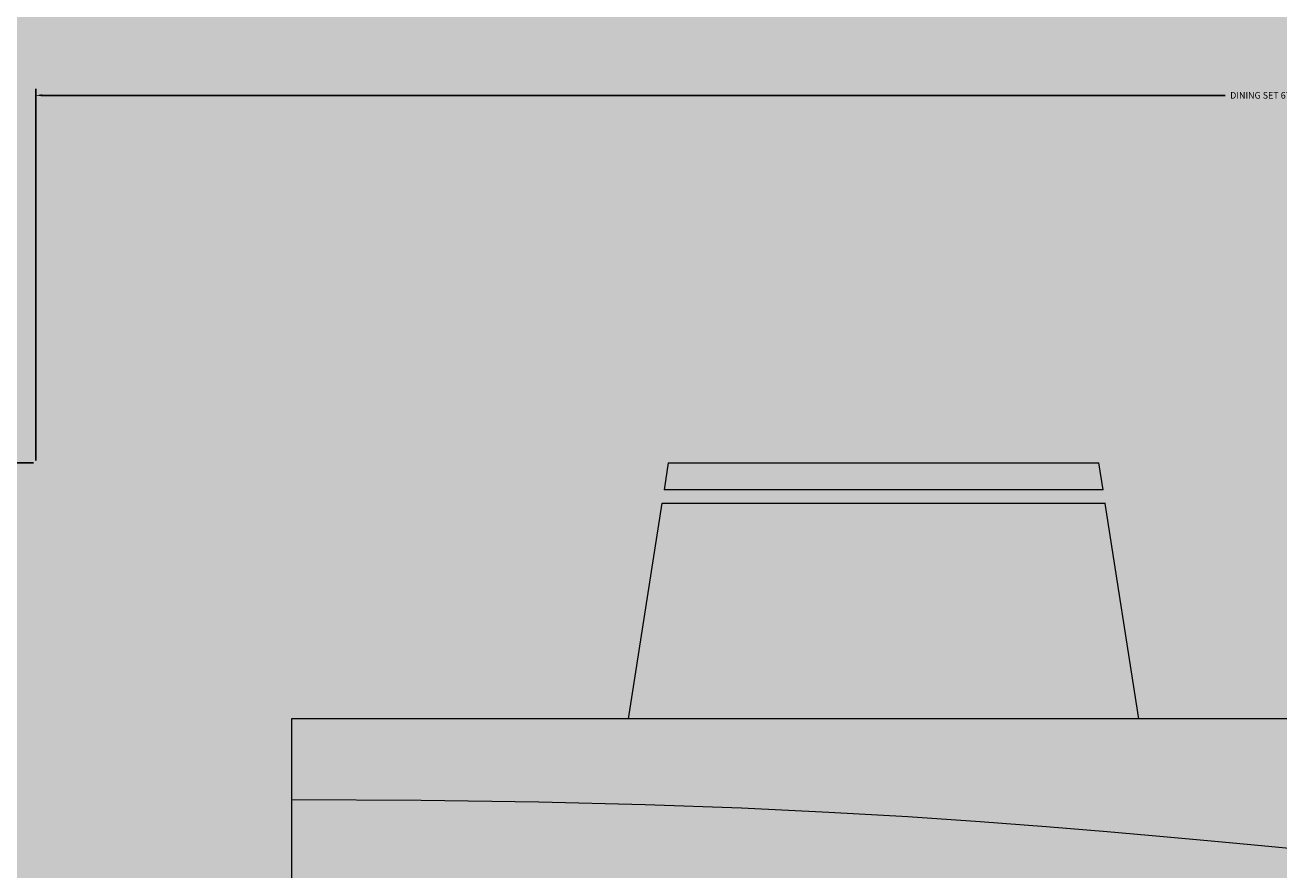
# Model space of a CAD drawing. Units: inches. Extents: x 3024 to 3952, y 1308 to 1863.
# Tile 9 of 29: x 3323 to 3357, y 1610 to 1633. Entities that reach past the tile are written whole.
import ezdxf

# ---------------------------------------------------------------- set-up
doc = ezdxf.new("R2010")
doc.units = ezdxf.units.IN
for name, color, linetype, lineweight in [('A-ANNO-DIMS', 2, 'Continuous', 18), ('A-FLOR-TILE-PATT', 7, 'Continuous', 13), ('A-FURN', 8, 'Continuous', 18), ('A-FURN-PATT', 9, 'Continuous', 13)]:
    doc.layers.add(name, color=color, linetype=linetype, lineweight=lineweight)
doc.layers.add('A-FLOR-PATT', color=254, linetype='Continuous', lineweight=13, true_color=0xfeeab9)
doc.styles.get("Standard").update_dxf_attribs({"font": 'arial.ttf'})
doc.dimstyles.get("Standard").update_dxf_attribs({"dimtxt": 0.18, "dimasz": 0.18, "dimexe": 0.18, "dimexo": 0.0625, "dimgap": 0.09, "dimtad": 0, "dimtih": 1, "dimtoh": 1, "dimdec": 4, "dimzin": 0, "dimdsep": 46, "dimtxsty": 'Standard', "dimcen": 0.09, "dimadec": 0, "dimazin": 0, "dimtfac": 1, "dimtdec": 4, "dimtofl": 0, "dimtmove": 0, "dimatfit": 3, "dimfxl": 1, "dimtolj": 1, "dimtzin": 0, "dimarcsym": 0})

# ---------------------------------------------------------------- blocks, each defined once
blk = doc.blocks.new('Dining Set - 36 x 72 in.')
for p, q in [((-22, 27.5), (-22.1562, 26.50042)), ((-22, 27.5), (-6, 27.5)), ((-5.8437, 26.49966), (-6, 27.5)), ((-5.8416, 26.5), (-22.1534, 26.5)), ((-22.2343, 26.00059), (-23.4847, 17.99762)), ((-22.2304, 26), (-5.7608, 26)), ((-4.5152, 17.99762), (-5.7655, 25.99926)), ((36, 18), (-36, 18)), ((-36, 18), (-36, -18))]:
    blk.add_line(p, q)
blk.add_lwpolyline([(-36, 15), (-31.1772, 14.97754), (-26.8079, 14.91406), (-22.8538, 14.81543), (-19.276, 14.6875), (-16.0362, 14.53613), (-13.0957, 14.36718), (-10.4159, 14.18652), (-7.9583, 14), (-5.6904, 13.81315), (-3.6035, 13.63021), (-1.6954, 13.45508), (0.0365, 13.29166), (1.5945, 13.14388)])
blk = doc.blocks.new('*D20')
at = {"layer": 'A-ANNO-DIMS', "color": 0, "lineweight": -2, "transparency": 16777216}
for p, q in [((3323.117, 1621.176), (3323.117, 1631.358)), ((3323.297, 1631.178), (3355.696, 1631.178)), ((3390.032, 1631.178), (3357.634, 1631.178)), ((3390.212, 1621.176), (3390.212, 1631.358))]:
    blk.add_line(p, q, dxfattribs=at)
at = {"layer": 'A-ANNO-DIMS', "color": 0, "transparency": 16777216}
for points in [[(3323.297, 1631.208), (3323.297, 1631.148), (3323.117, 1631.178)], [(3390.032, 1631.208), (3390.032, 1631.148), (3390.212, 1631.178)]]:
    blk.add_solid(points, dxfattribs=at)
at = {"layer": 'Defpoints', "color": 0, "transparency": 16777216}
for p in [(3390.212, 1631.178), (3323.117, 1621.114), (3390.212, 1621.114)]:
    blk.add_point(p, dxfattribs=at)
at = {"layer": 'A-ANNO-DIMS', "color": 0, "transparency": 16777216, "insert": (3356.665, 1631.178), "char_height": 0.18, "attachment_point": 5}
blk.add_mtext('\\A1;DINING SET 67', dxfattribs=at)
blk = doc.blocks.new('*D21')
at = {"layer": 'A-ANNO-DIMS', "color": 0, "lineweight": -2, "transparency": 16777216}
for p, q in [((3323.055, 1621.114), (3312.873, 1621.114)), ((3313.053, 1620.934), (3313.053, 1601.018)), ((3313.053, 1580.742), (3313.053, 1600.657)), ((3323.055, 1580.562), (3312.873, 1580.562))]:
    blk.add_line(p, q, dxfattribs=at)
at = {"layer": 'A-ANNO-DIMS', "color": 0, "transparency": 16777216}
for points in [[(3313.023, 1620.934), (3313.083, 1620.934), (3313.053, 1621.114)], [(3313.023, 1580.742), (3313.083, 1580.742), (3313.053, 1580.562)]]:
    blk.add_solid(points, dxfattribs=at)
at = {"layer": 'Defpoints', "color": 0, "transparency": 16777216}
for p in [(3313.053, 1621.114), (3323.117, 1621.114), (3323.117, 1580.562)]:
    blk.add_point(p, dxfattribs=at)
at = {"layer": 'A-ANNO-DIMS', "color": 0, "transparency": 16777216, "insert": (3313.053, 1600.838), "char_height": 0.18, "attachment_point": 5}
blk.add_mtext('\\A1;41', dxfattribs=at)

msp = doc.modelspace()

# ---------------------------------------------------------------- hatches: boundary and pattern name
at = {"layer": 'A-FLOR-PATT', "transparency": 33554528}
h = msp.add_hatch(color=256, dxfattribs=at)
h.dxf.hatch_style = 1
h.paths.add_polyline_path([(3460.764, 1688.6064), (3412.764, 1688.6064), (3412.764, 1694.6064), (3460.764, 1694.6064), (3460.764, 1778.6064), (3406.764, 1778.6064), (3406.764, 1759.9514), (3318.2981, 1759.9514), (3318.2981, 1658.6064), (3322.5356, 1658.6064), (3322.5356, 1652.6064), (3292.764, 1652.6064), (3292.764, 1778.6064), (3106.764, 1778.6064), (3106.764, 1628.6064), (3172.764, 1628.6064), (3172.764, 1532.6064), (3166.764, 1532.6064), (3166.764, 1628.6064), (3106.764, 1628.6064), (3106.764, 1356.8452), (3202.812, 1356.8452), (3202.812, 1354.2534), (3202.812, 1353.8388), (3202.812, 1351.1212), (3202.812, 1347.8452), (3277.764, 1347.8452), (3277.764, 1353.8452), (3277.764, 1356.8452), (3277.764, 1442.6064), (3460.764, 1442.6064)])
h.paths.add_polyline_path([(3216.238, 1527.2064), (3216.238, 1491.2064), (3214.663, 1491.2064), (3214.663, 1491.2409, -0.3966224), (3180.243, 1526.6064), (3163.0285, 1526.6064), (3163.0285, 1531.1064), (3161.716, 1531.1064), (3161.716, 1561.1064), (3163.0285, 1561.1064), (3163.0285, 1531.1064), (3163.0285, 1526.6064), (3180.243, 1526.6064, 0.3966224), (3214.663, 1491.2409), (3214.663, 1527.2064)], flags=16)
h.paths.add_polyline_path([(3227.364, 1649.8972), (3191.364, 1649.8972), (3191.364, 1651.4722), (3227.364, 1651.4722)], flags=16)
h.paths.add_polyline_path([(3323.1172, 1606.7362), (3323.8545, 1606.8514), (3323.8545, 1594.8241), (3323.1172, 1594.9393)], flags=16)
h.paths.add_polyline_path([(3324.2232, 1606.909), (3330.1216, 1607.8307), (3330.1216, 1614.1093), (3339.3495, 1614.1093), (3340.2711, 1620.0078), (3352.4136, 1620.0078), (3353.3353, 1614.1093), (3359.9941, 1614.1093), (3360.9157, 1620.0078), (3373.0582, 1620.0078), (3373.9799, 1614.1093), (3383.2077, 1614.1093), (3383.2077, 1607.8307), (3389.1062, 1606.909), (3389.1062, 1594.7665), (3383.2077, 1593.8449), (3383.2077, 1587.5663), (3373.9799, 1587.5663), (3373.0583, 1581.6678), (3360.9157, 1581.6678), (3359.9941, 1587.5663), (3353.3353, 1587.5663), (3352.4136, 1581.6678), (3340.2711, 1581.6678), (3339.3495, 1587.5663), (3330.1216, 1587.5663), (3330.1216, 1593.8449), (3324.2232, 1594.7665)], flags=16)
h.paths.add_polyline_path([(3236.1584, 1693.1064), (3236.1584, 1723.1064), (3237.4709, 1723.1064), (3237.4709, 1693.1064)], flags=16)
h.paths.add_polyline_path([(3373.2158, 1600.6847), (3373.7965, 1600.7303), (3374.3268, 1600.7874), (3374.8132, 1600.8531), (3375.2621, 1600.9247), (3375.6801, 1600.9991), (3376.0736, 1601.0735), (3376.6855, 1601.19), (3377.366, 1601.3023), (3378.0667, 1601.3814), (3378.8026, 1601.4123), (3379.5865, 1601.3839), (3380.4537, 1601.2948), (3381.301, 1601.1717), (3382.0317, 1601.0433), (3382.4398, 1600.9607), (3382.6252, 1600.9201), (3382.919, 1600.8507), (3382.9044, 1600.8531), (3382.842, 1600.8678), (3382.7541, 1600.8896), (3382.6252, 1600.9201), (3382.4398, 1600.9607), (3382.1868, 1601.0119), (3381.8738, 1601.0711), (3381.5125, 1601.1346), (3381.1149, 1601.1988), (3380.6928, 1601.2601), (3380.2581, 1601.3149), (3379.8226, 1601.3597), (3379.3984, 1601.3908), (3378.9944, 1601.4054), (3378.6092, 1601.4042), (3378.2384, 1601.3886), (3377.8777, 1601.36), (3377.5227, 1601.32), (3377.1691, 1601.2698), (3376.8127, 1601.211), (3376.4491, 1601.145), (3376.0736, 1601.0735), (3375.4177, 1600.9494), (3374.5542, 1600.8119), (3373.5044, 1600.6988)], flags=0)
h.paths.add_polyline_path([(3380.0253, 1596.7351), (3380.499, 1596.6659), (3380.9706, 1596.6119), (3381.4375, 1596.5791), (3381.8971, 1596.5736), (3382.5886, 1596.6167), (3382.7848, 1596.6692), (3382.1465, 1596.5706), (3381.236, 1596.5815), (3380.3199, 1596.6865)], flags=0)
h.paths.add_polyline_path([(3369.6414, 1603.9617), (3370.1589, 1604.0021), (3370.6218, 1604.0539), (3371.0335, 1604.1173), (3371.3978, 1604.1921), (3371.7181, 1604.2785), (3371.9984, 1604.3761), (3372.2441, 1604.483), (3372.4611, 1604.5972), (3372.655, 1604.7163), (3372.8317, 1604.8384), (3372.9968, 1604.9611), (3373.3703, 1605.2455), (3373.8426, 1605.5328), (3374.4624, 1605.7539), (3375.1058, 1605.8302), (3375.7221, 1605.8261), (3376.4109, 1605.76), (3377.1534, 1605.6376), (3377.8945, 1605.473), (3378.1382, 1605.409), (3377.7394, 1605.5074), (3377.3509, 1605.5937), (3376.9704, 1605.6677), (3376.5999, 1605.7288), (3376.2417, 1605.7762), (3375.8979, 1605.8092), (3375.5707, 1605.8271), (3375.2621, 1605.8291), (3374.9745, 1605.8146), (3374.7092, 1605.7832), (3374.4647, 1605.7359), (3374.239, 1605.6742), (3374.0298, 1605.5996), (3373.835, 1605.5134), (3373.6525, 1605.4171), (3373.4801, 1605.3123), (3373.3156, 1605.2002), (3373.1562, 1605.0825), (3372.7603, 1604.781), (3372.236, 1604.4588), (3371.5738, 1604.2283), (3370.8493, 1604.0794), (3369.9262, 1603.976)], flags=0)
h.paths.add_polyline_path([(3366.7533, 1606.5832), (3367.1713, 1606.5519), (3367.5378, 1606.5374), (3367.8568, 1606.5394), (3368.1325, 1606.5573), (3368.3694, 1606.5903), (3368.5717, 1606.6377), (3368.7438, 1606.6988), (3368.89, 1606.7728), (3369.0146, 1606.8591), (3369.121, 1606.9568), (3369.2094, 1607.0646), (3369.2792, 1607.181), (3369.3295, 1607.3046), (3369.3596, 1607.4339), (3369.3688, 1607.5676), (3369.3565, 1607.7042), (3369.3218, 1607.8422), (3369.2649, 1607.9804), (3369.1893, 1608.1187), (3369.0993, 1608.2569), (3368.9992, 1608.3952), (3368.8934, 1608.5334), (3368.7861, 1608.6717), (3368.6817, 1608.8099), (3368.4212, 1609.1804), (3368.2685, 1609.7106), (3368.4883, 1610.1814), (3369.0537, 1610.4604), (3369.6717, 1610.5097), (3370.2812, 1610.3612), (3370.4805, 1610.2968), (3370.1882, 1610.3839), (3369.9284, 1610.4472), (3369.6905, 1610.4842), (3369.4662, 1610.4933), (3369.2555, 1610.4765), (3369.0608, 1610.4367), (3368.884, 1610.3767), (3368.7274, 1610.2994), (3368.5931, 1610.2077), (3368.4833, 1610.1045), (3368.4002, 1609.9927), (3368.3451, 1609.8747), (3368.3166, 1609.7517), (3368.3127, 1609.6244), (3368.331, 1609.4935), (3368.3696, 1609.3597), (3368.4261, 1609.2237), (3368.4985, 1609.0863), (3368.5845, 1608.9482), (3368.6817, 1608.8099), (3368.7861, 1608.6717), (3368.8934, 1608.5334), (3368.9992, 1608.3952), (3369.0993, 1608.2569), (3369.3398, 1607.8876), (3369.3941, 1607.2896), (3368.9774, 1606.7817), (3368.3928, 1606.5742), (3367.7162, 1606.5303), (3367.0044, 1606.5585)], flags=0)
h.paths.add_polyline_path([(3362.1859, 1610.2589), (3362.5478, 1610.2845), (3362.8348, 1610.3275), (3363.0585, 1610.3863), (3363.2303, 1610.4595), (3363.3619, 1610.5457), (3363.463, 1610.6432), (3363.5376, 1610.7502), (3363.5876, 1610.8643), (3363.6153, 1610.9834), (3363.6229, 1611.1055), (3363.6125, 1611.2283), (3363.5861, 1611.3496), (3363.5462, 1611.4673), (3363.4949, 1611.5797), (3363.4358, 1611.6871), (3363.3723, 1611.7902), (3363.3081, 1611.8897), (3363.2468, 1611.9863), (3363.192, 1612.0808), (3363.0258, 1612.4261), (3363.3371, 1612.8672), (3363.9008, 1612.9782), (3364.4822, 1612.9641), (3365.1098, 1612.9074), (3365.328, 1612.8805), (3364.9615, 1612.9208), (3364.6426, 1612.9496), (3364.3668, 1612.9669), (3364.1299, 1612.9726), (3363.9276, 1612.9669), (3363.7555, 1612.9496), (3363.6093, 1612.9208), (3363.4848, 1612.8805), (3363.3782, 1612.8289), (3363.2889, 1612.7672), (3363.2169, 1612.6969), (3363.1622, 1612.6193), (3363.1247, 1612.5361), (3363.1046, 1612.4484), (3363.1017, 1612.358), (3363.1161, 1612.266), (3363.1472, 1612.1738), (3363.192, 1612.0808), (3363.2468, 1611.9863), (3363.3081, 1611.8897), (3363.3723, 1611.7902), (3363.4358, 1611.6871), (3363.6363, 1611.323), (3363.5979, 1610.7003), (3363.0863, 1610.3651), (3362.3983, 1610.2622)], flags=0)
h.paths.add_polyline_path([(3352.356, 1581.2991), (3352.2408, 1580.5618), (3340.4439, 1580.5618), (3340.3287, 1581.2991)], flags=16)
h.paths.add_polyline_path([(3340.4439, 1621.1137), (3352.2408, 1621.1137), (3352.356, 1620.3764), (3340.3287, 1620.3764)], flags=16)
h.paths.add_polyline_path([(3278.4282, 1504.7424), (3290.3831, 1504.7424), (3290.3831, 1502.7499), (3291.0473, 1502.7499), (3291.0473, 1494.7799), (3290.3831, 1494.7799), (3290.3831, 1494.1158), (3291.0473, 1494.1158), (3291.0473, 1486.1458), (3290.3831, 1486.1458), (3290.3831, 1484.1533), (3291.0473, 1484.1533), (3291.0473, 1483.4892, -0.0909091), (3291.0473, 1468.8776), (3291.0473, 1468.2135), (3290.3831, 1468.2135), (3290.3831, 1464.8926), (3278.4282, 1464.8926), (3278.4282, 1472.8626), (3277.764, 1473.5268), (3277.764, 1478.84), (3278.4282, 1479.5042)], flags=16)
h.paths.add_polyline_path([(3278.7603, 1504.4103), (3290.051, 1504.4103), (3290.051, 1465.2247), (3278.7603, 1465.2247)], flags=0)
h.paths.add_polyline_path([(3123.904, 1600.7821), (3117.9039, 1602.7821), (3117.9039, 1599.7821), (3119.4039, 1599.7821), (3119.4039, 1596.7821), (3118.4039, 1596.7821), (3118.4039, 1598.7821), (3117.9039, 1598.7821), (3117.9039, 1596.2821), (3109.9039, 1596.2821), (3109.9039, 1617.2821), (3117.9039, 1617.2821), (3117.9039, 1610.7821), (3123.9038, 1612.7821, -0.7025712), (3137.9039, 1606.7822, -0.7025621)], flags=16)
h.paths.add_polyline_path([(3123.9039, 1602.7822), (3123.9039, 1610.7822, -0.7345333), (3136.9039, 1606.7822, -0.7345297)], flags=0)
h.paths.add_polyline_path([(3177.972, 1689.6473), (3109.2405, 1689.6473), (3109.2405, 1741.1959), (3177.972, 1741.1959)], flags=16)
h.paths.add_polyline_path([(3373.0006, 1581.2991), (3372.8854, 1580.5618), (3361.0885, 1580.5618), (3360.9733, 1581.2991)], flags=16)
h.paths.add_polyline_path([(3361.0885, 1621.1137), (3372.8854, 1621.1137), (3373.0006, 1620.3764), (3360.9733, 1620.3764)], flags=16)
h.paths.add_polyline_path([(3116.9039, 1598.2821, -0.4142136), (3116.1539, 1597.2821), (3111.9039, 1597.2821, -0.4142136), (3110.9039, 1598.0321), (3110.9039, 1615.2821, -0.4142136), (3111.6539, 1616.2821), (3115.9039, 1616.2821, -0.4142136), (3116.9039, 1615.5321)], flags=0)
h.paths.add_polyline_path([(3121.6122, 1728.1369), (3121.6122, 1696.5205), (3110.2715, 1696.5205), (3110.2715, 1714.3906), (3121.6122, 1714.3906), (3121.6122, 1716.4526), (3110.2715, 1716.4526), (3110.2715, 1734.3228), (3123.3304, 1734.3228), (3123.3304, 1729.8552), (3134.6711, 1741.1959), (3134.6711, 1728.1369)], flags=0)
h.paths.add_polyline_path([(3389.4748, 1606.8514), (3390.2122, 1606.7362), (3390.2122, 1594.9393), (3389.4748, 1594.8241)], flags=16)
h.paths.add_polyline_path([(3257.6842, 1762.8281), (3259.6842, 1768.8281), (3256.6842, 1768.8281), (3256.6842, 1767.3281), (3253.6842, 1767.3281), (3253.6842, 1768.3281), (3255.6842, 1768.3281), (3255.6842, 1768.8281), (3253.1842, 1768.8281), (3253.1842, 1776.8281), (3274.1842, 1776.8281), (3274.1842, 1768.8281), (3267.6842, 1768.8281), (3269.6842, 1762.8282, -0.7025712), (3263.6843, 1748.8282, -0.7025621)], flags=16)
h.paths.add_polyline_path([(3259.6842, 1762.8281), (3267.6843, 1762.8281, -0.7345333), (3263.6842, 1749.8282, -0.7345297)], flags=0)
h.paths.add_polyline_path([(3411.264, 1715.6064), (3411.264, 1716.9189), (3441.264, 1716.9189), (3441.264, 1715.6064)], flags=16)
h.paths.add_polyline_path([(3178.3806, 1449.1876), (3178.3806, 1397.639), (3109.6491, 1397.639), (3109.6491, 1449.1876)], flags=16)
h.paths.add_polyline_path([(3397.1501, 1541.7146), (3419.6183, 1541.7146), (3419.6183, 1496.7783), (3397.1501, 1496.7783)], flags=16)
h.paths.add_polyline_path([(3254.1842, 1770.5781), (3254.1842, 1774.8281, -0.4142136), (3254.9342, 1775.8281), (3272.1842, 1775.8281, -0.4142136), (3273.1842, 1775.0781), (3273.1842, 1770.8281, -0.4142136), (3272.4342, 1769.8281), (3255.1842, 1769.8281, -0.4142136)], flags=0)
h.paths.add_polyline_path([(3403.672, 1500.7601), (3403.6016, 1500.3997), (3403.5328, 1500.0441), (3403.4662, 1499.6867), (3403.4027, 1499.3226), (3403.3464, 1498.9532), (3403.3025, 1498.5811), (3403.2759, 1498.2091), (3403.2714, 1497.8401), (3403.3064, 1497.2813), (3403.3491, 1497.1219), (3403.2689, 1497.6395), (3403.2778, 1498.3719), (3403.3635, 1499.0984), (3403.4889, 1499.8168), (3403.6016, 1500.3997), (3403.672, 1500.7601), (3403.744, 1501.1315), (3403.817, 1501.5205), (3403.891, 1501.9336), (3403.9656, 1502.3769), (3404.0404, 1502.8572), (3404.115, 1503.3786), (3404.2264, 1504.2311), (3404.2571, 1504.5223), (3404.1552, 1503.6598), (3404.0063, 1502.6193), (3403.8604, 1501.7518), (3403.744, 1501.1315)], flags=0)
h.paths.add_polyline_path([(3406.5868, 1505.0416), (3406.6121, 1504.5236), (3406.6492, 1504.0526), (3406.6956, 1503.624), (3406.7491, 1503.2333), (3406.8072, 1502.8759), (3406.8676, 1502.5473), (3406.9281, 1502.243), (3407.0268, 1501.7597), (3407.1416, 1501.1368), (3407.2087, 1500.3904), (3407.1804, 1499.6703), (3407.1078, 1498.9956), (3407.0074, 1498.3199), (3406.8809, 1497.6059), (3406.7403, 1496.9627), (3406.7418, 1496.9824), (3406.7491, 1497.0249), (3406.8229, 1497.3409), (3406.8364, 1497.4025), (3406.878, 1497.6078), (3406.9261, 1497.8614), (3406.9777, 1498.1526), (3407.0298, 1498.4712), (3407.0797, 1498.8068), (3407.1243, 1499.149), (3407.1607, 1499.4874), (3407.1859, 1499.8115), (3407.1978, 1500.1137), (3407.1969, 1500.3962), (3407.1841, 1500.6642), (3407.1609, 1500.9225), (3407.1284, 1501.1761), (3407.0876, 1501.43), (3407.0398, 1501.6891), (3406.9862, 1501.9585), (3406.8832, 1502.4628), (3406.7712, 1503.0713), (3406.6657, 1503.8424), (3406.5924, 1504.7735)], flags=0)
h.paths.add_polyline_path([(3409.2517, 1507.8962), (3409.2752, 1507.4282), (3409.3079, 1507.0076), (3409.3501, 1506.6314), (3409.4015, 1506.2969), (3409.4624, 1506.0009), (3409.5326, 1505.7406), (3409.6119, 1505.5128), (3409.6988, 1505.3131), (3409.7915, 1505.1368), (3409.8883, 1504.9792), (3409.9875, 1504.8356), (3410.0872, 1504.7015), (3410.1859, 1504.572), (3410.4508, 1504.2132), (3410.7205, 1503.6035), (3410.8059, 1502.8824), (3410.7619, 1502.0875), (3410.6122, 1501.2299), (3410.4402, 1500.6169), (3410.2538, 1500.0031), (3410.0536, 1499.3219), (3409.9909, 1499.0812), (3410.1761, 1499.7472), (3410.3596, 1500.3513), (3410.4512, 1500.6561), (3410.5312, 1500.9412), (3410.6013, 1501.226), (3410.6614, 1501.512), (3410.7111, 1501.7964), (3410.7496, 1502.0763), (3410.7764, 1502.3489), (3410.7909, 1502.6114), (3410.7926, 1502.8608), (3410.7808, 1503.0944), (3410.7553, 1503.31), (3410.7169, 1503.5087), (3410.6667, 1503.6921), (3410.6061, 1503.8621), (3410.5361, 1504.0203), (3410.4578, 1504.1686), (3410.3726, 1504.3088), (3410.2815, 1504.4424), (3410.1859, 1504.572), (3410.0872, 1504.7015), (3409.859, 1505.0083), (3409.5943, 1505.5117), (3409.4266, 1506.1336), (3409.324, 1506.8011), (3409.2586, 1507.6407)], flags=0)
h.paths.add_polyline_path([(3411.4914, 1510.5878), (3411.4432, 1510.1586), (3411.4054, 1509.775), (3411.38, 1509.4354), (3411.3681, 1509.1376), (3411.3698, 1508.8784), (3411.3843, 1508.6542), (3411.4112, 1508.4618), (3411.4497, 1508.2974), (3411.4994, 1508.1575), (3411.5595, 1508.0388), (3411.6296, 1507.9375), (3411.7097, 1507.851), (3411.802, 1507.7792), (3411.9096, 1507.7225), (3412.0353, 1507.6817), (3412.1821, 1507.6572), (3412.3528, 1507.6496), (3412.5505, 1507.6597), (3412.778, 1507.6879), (3413.0364, 1507.7341), (3413.3194, 1507.7955), (3413.6188, 1507.8687), (3413.9264, 1507.95), (3414.234, 1508.036), (3414.5333, 1508.1232), (3414.8163, 1508.208), (3415.0747, 1508.287), (3415.3023, 1508.3569), (3415.5007, 1508.4158), (3415.6733, 1508.4617), (3416.1158, 1508.5538), (3416.512, 1508.2591), (3416.716, 1507.6581), (3416.61, 1507.0003), (3416.3052, 1506.3411), (3415.8928, 1505.618), (3415.7339, 1505.3633), (3415.9914, 1505.791), (3416.201, 1506.1583), (3416.3666, 1506.4739), (3416.4925, 1506.7462), (3416.5828, 1506.9838), (3416.6413, 1507.1949), (3416.6725, 1507.3883), (3416.6799, 1507.5705), (3416.6662, 1507.7417), (3416.6339, 1507.9), (3416.5851, 1508.0436), (3416.5223, 1508.1709), (3416.4478, 1508.28), (3416.3639, 1508.3692), (3416.273, 1508.4368), (3416.1765, 1508.4815), (3416.0718, 1508.5047), (3415.9553, 1508.5079), (3415.8237, 1508.493), (3415.6733, 1508.4617), (3415.5007, 1508.4158), (3415.3327, 1508.3659), (3414.6495, 1508.157), (3414.0606, 1507.9855), (3413.4456, 1507.8229), (3412.8838, 1507.701), (3412.5505, 1507.6597), (3412.0748, 1507.6354), (3411.595, 1507.8883), (3411.398, 1508.4429), (3411.3624, 1508.9927), (3411.3854, 1509.5711), (3411.4578, 1510.3071)], flags=0)
h.paths.add_polyline_path([(3135.0797, 1449.1876), (3135.0797, 1436.1286), (3122.0208, 1436.1286), (3122.0208, 1404.5122), (3110.6801, 1404.5122), (3110.6801, 1422.3823), (3122.0208, 1422.3823), (3122.0208, 1424.4443), (3110.6801, 1424.4443), (3110.6801, 1442.3145), (3123.739, 1442.3145), (3123.739, 1437.8469)], flags=0)
h.paths.add_polyline_path([(3416.4944, 1514.2949), (3416.4837, 1513.8511), (3416.4893, 1513.4867), (3416.5102, 1513.1926), (3416.5451, 1512.9593), (3416.5929, 1512.7775), (3416.6524, 1512.6379), (3416.7224, 1512.531), (3416.8017, 1512.4488), (3416.8886, 1512.3882), (3416.9813, 1512.3476), (3417.0781, 1512.3251), (3417.1773, 1512.3189), (3417.277, 1512.3274), (3417.3757, 1512.3488), (3417.4713, 1512.3813), (3417.5627, 1512.4229), (3417.65, 1512.471), (3417.7338, 1512.5225), (3417.8146, 1512.5747), (3417.8931, 1512.6245), (3417.9699, 1512.6691), (3418.2968, 1512.8265), (3418.6505, 1512.4645), (3418.7037, 1511.9342), (3418.6693, 1511.3839), (3418.6076, 1510.8228), (3418.5777, 1510.5927), (3418.6197, 1510.9333), (3418.6525, 1511.2311), (3418.6759, 1511.4903), (3418.6899, 1511.7144), (3418.6946, 1511.9069), (3418.6899, 1512.0713), (3418.6759, 1512.2112), (3418.6525, 1512.33), (3418.6197, 1512.4311), (3418.5778, 1512.5177), (3418.5276, 1512.5903), (3418.4705, 1512.6488), (3418.4075, 1512.6933), (3418.3399, 1512.7237), (3418.2686, 1512.7401), (3418.1951, 1512.7424), (3418.1204, 1512.7307), (3418.0455, 1512.7055), (3417.9792, 1512.6736), (3417.65, 1512.471), (3417.5627, 1512.4229), (3417.4713, 1512.3813), (3417.3757, 1512.3488), (3417.277, 1512.3274), (3416.878, 1512.2936), (3416.5757, 1512.7549), (3416.492, 1513.3145), (3416.4808, 1514.0384)], flags=0)
h.paths.add_polyline_path([(3392.8223, 1481.9454), (3396.7707, 1481.9454), (3396.7707, 1480.9201), (3428.3585, 1480.9201), (3428.3585, 1481.9454), (3432.3069, 1481.9454), (3432.3069, 1464.8354, -0.266667), (3392.8223, 1464.8354)], flags=16)
h.paths.add_polyline_path([(3431.203, 1547.5428), (3450.8613, 1547.5428, -0.1904762), (3450.8614, 1484.031), (3431.203, 1484.031), (3431.203, 1488.5675), (3432.3809, 1488.5675), (3432.3809, 1543.0062), (3431.203, 1543.0062)], flags=16)
h.paths.add_polyline_path([(3451.9233, 1524.86, -0.0496282), (3451.9233, 1506.7138), (3446.7921, 1506.7138), (3446.7921, 1524.86)], flags=0)
h.paths.add_polyline_path([(3460.764, 1436.6064), (3277.764, 1436.6064), (3277.764, 1356.8452), (3277.764, 1353.8452), (3460.764, 1353.8452)], flags=17)
h.paths.add_polyline_path([(3121.3033, 1577.378), (3153.693, 1577.378), (3153.693, 1586.6752), (3121.3033, 1586.6752)], flags=24)
h.paths.add_polyline_path([(3164.1457, 1464.1276), (3210.4801, 1464.1276), (3210.4801, 1473.4247), (3164.1457, 1473.4247)], flags=24)
h.paths.add_polyline_path([(3343.1909, 1505.8863), (3373.7236, 1505.8863), (3373.7236, 1515.1773), (3343.1909, 1515.1773)], flags=24)
h.paths.add_polyline_path([(3337.6353, 1564.2926), (3370.0189, 1564.2926), (3370.0189, 1573.5836), (3337.6353, 1573.5836)], flags=24)
h.paths.add_polyline_path([(3419.204, 1753.8578), (3453.3997, 1753.8578), (3453.3997, 1762.9956), (3419.204, 1762.9956)], flags=24)
h.paths.add_polyline_path([(3341.2523, 1701.0246), (3381.0761, 1701.0246), (3381.0761, 1710.3156), (3341.2523, 1710.3156)], flags=24)
h.paths.add_polyline_path([(3245.8895, 1726.2997), (3278.2793, 1726.2997), (3278.2793, 1735.5968), (3245.8895, 1735.5968)], flags=24)
h.paths.add_polyline_path([(3128.8045, 1668.6736), (3175.1389, 1668.6736), (3175.1389, 1677.9707), (3128.8045, 1677.9707)], flags=24)
h.paths.add_polyline_path([(3345.9997, 1396.0062), (3389.09, 1396.0062), (3389.09, 1405.3033), (3345.9997, 1405.3033)], flags=24)
at = {"layer": 'A-FLOR-TILE-PATT', "transparency": 33554569}
h = msp.add_hatch(dxfattribs=at)
h.set_pattern_fill('ANGLE', color=256, scale=2)
h.set_pattern_definition([(0, (0, 0), (0, 13.97), [10.16, -3.81]), (90, (0, 0), (-13.97, 9e-16), [10.16, -3.81])])
h.paths.add_polyline_path([(3292.764, 1778.6064), (3232.764, 1778.6064), (3232.764, 1694.6064), (3236.1584, 1694.6064), (3236.1584, 1723.1064), (3237.4709, 1723.1064), (3237.4709, 1723.0777, -0.3870039), (3266.1209, 1694.6064), (3292.764, 1694.6064)])
h.paths.add_polyline_path([(3263.6843, 1748.8282, -0.7025621), (3257.6842, 1762.8281), (3259.6842, 1768.8281), (3256.6842, 1768.8281), (3256.6842, 1767.3281), (3253.6842, 1767.3281), (3253.6842, 1768.3281), (3255.6842, 1768.3281), (3255.6842, 1768.8281), (3253.1842, 1768.8281), (3253.1842, 1776.8281), (3274.1842, 1776.8281), (3274.1842, 1768.8281), (3267.6842, 1768.8281), (3269.6842, 1762.8282, -0.7025712)], flags=16)
h.paths.add_polyline_path([(3263.6842, 1749.8282, -0.7345297), (3259.6842, 1762.8281), (3267.6843, 1762.8281, -0.7345333)], flags=0)
h.paths.add_polyline_path([(3255.1842, 1769.8281, -0.4142136), (3254.1842, 1770.5781), (3254.1842, 1774.8281, -0.4142136), (3254.9342, 1775.8281), (3272.1842, 1775.8281, -0.4142136), (3273.1842, 1775.0781), (3273.1842, 1770.8281, -0.4142136), (3272.4342, 1769.8281)], flags=0)
h.paths.add_polyline_path([(3460.764, 1436.6064), (3277.764, 1436.6064), (3277.764, 1356.8452), (3277.764, 1353.8452), (3460.764, 1353.8452)])
h.paths.add_polyline_path([(3166.764, 1628.6064), (3106.764, 1628.6064), (3106.764, 1532.6064), (3133.066, 1532.6064, -0.3870039), (3161.716, 1561.0777), (3161.716, 1561.1064), (3163.0285, 1561.1064), (3163.0285, 1532.6064), (3166.764, 1532.6064)])
h.paths.add_polyline_path([(3123.904, 1600.7821), (3117.9039, 1602.7821), (3117.9039, 1599.7821), (3119.4039, 1599.7821), (3119.4039, 1596.7821), (3118.4039, 1596.7821), (3118.4039, 1598.7821), (3117.9039, 1598.7821), (3117.9039, 1596.2821), (3109.9039, 1596.2821), (3109.9039, 1617.2821), (3117.9039, 1617.2821), (3117.9039, 1610.7821), (3123.9038, 1612.7821, -0.7025712), (3137.9039, 1606.7822, -0.7025621)], flags=16)
h.paths.add_polyline_path([(3123.9039, 1602.7822), (3123.9039, 1610.7822, -0.7345333), (3136.9039, 1606.7822, -0.7345297)], flags=0)
h.paths.add_polyline_path([(3116.1539, 1597.2821), (3111.9039, 1597.2821, -0.4142136), (3110.9039, 1598.0321), (3110.9039, 1615.2821, -0.4142136), (3111.6539, 1616.2821), (3115.9039, 1616.2821, -0.4142136), (3116.9039, 1615.5321), (3116.9039, 1598.2821, -0.4142136)], flags=0)
h.paths.add_polyline_path([(3245.8895, 1726.2997), (3278.2793, 1726.2997), (3278.2793, 1735.5968), (3245.8895, 1735.5968)], flags=24)
h.paths.add_polyline_path([(3345.9997, 1396.0062), (3389.09, 1396.0062), (3389.09, 1405.3033), (3345.9997, 1405.3033)], flags=24)
h.paths.add_polyline_path([(3121.3033, 1577.378), (3153.693, 1577.378), (3153.693, 1586.6752), (3121.3033, 1586.6752)], flags=24)
at = {"layer": 'A-FURN-PATT', "transparency": 33554511}
h = msp.add_hatch(color=256, dxfattribs=at)
h.dxf.hatch_style = 1
h.paths.add_polyline_path([(3373.0582, 1620.0078), (3360.9157, 1620.0078), (3359.9941, 1614.1093), (3373.9799, 1614.1093)])
h.paths.add_polyline_path([(3372.8854, 1621.1137), (3361.0885, 1621.1137), (3360.9733, 1620.3764), (3373.0006, 1620.3764)])
h.paths.add_polyline_path([(3389.1062, 1606.909), (3383.2077, 1607.8307), (3383.2077, 1593.8449), (3389.1062, 1594.7665)])
h.paths.add_polyline_path([(3390.2122, 1606.7362), (3389.4748, 1606.8514), (3389.4748, 1594.8241), (3390.2122, 1594.9393)])
h.paths.add_polyline_path([(3373.9799, 1587.5663), (3359.9941, 1587.5663), (3360.9157, 1581.6678), (3373.0583, 1581.6678)])
h.paths.add_polyline_path([(3373.0006, 1581.2991), (3360.9733, 1581.2991), (3361.0885, 1580.5618), (3372.8854, 1580.5618)])
h.paths.add_polyline_path([(3353.3353, 1587.5663), (3339.3495, 1587.5663), (3340.2711, 1581.6678), (3352.4136, 1581.6678)])
h.paths.add_polyline_path([(3352.356, 1581.2991), (3340.3287, 1581.2991), (3340.4439, 1580.5618), (3352.2408, 1580.5618)])
h.paths.add_polyline_path([(3330.1216, 1607.8307), (3324.2232, 1606.909), (3324.2232, 1594.7665), (3330.1216, 1593.8449)])
h.paths.add_polyline_path([(3323.8545, 1606.8514), (3323.1172, 1606.7362), (3323.1172, 1594.9393), (3323.8545, 1594.8241)])
h.paths.add_polyline_path([(3352.4136, 1620.0078), (3340.2711, 1620.0078), (3339.3495, 1614.1093), (3353.3353, 1614.1093)])
h.paths.add_polyline_path([(3352.2408, 1621.1137), (3340.4439, 1621.1137), (3340.3287, 1620.3764), (3352.356, 1620.3764)])
at = {"layer": 'A-FURN-PATT', "transparency": 33554600}
h = msp.add_hatch(color=256, dxfattribs=at)
h.dxf.hatch_style = 1
h.paths.add_polyline_path([(3363.5462, 1611.4673), (3363.4949, 1611.5797), (3363.4358, 1611.6871), (3363.3723, 1611.7902), (3363.2557, 1611.9708), (3363.16, 1612.1359), (3363.1003, 1612.3129), (3363.1061, 1612.4946), (3363.1815, 1612.6623), (3363.3264, 1612.8038), (3363.5397, 1612.9071), (3363.7555, 1612.9496), (3363.9276, 1612.9669), (3364.1299, 1612.9726), (3364.3668, 1612.9669), (3364.6426, 1612.9496), (3364.9615, 1612.9208), (3365.328, 1612.8805), (3365.7471, 1612.8287), (3366.2271, 1612.7662), (3366.7769, 1612.6936), (3367.4055, 1612.6117), (3368.1221, 1612.5211), (3368.9354, 1612.4225), (3369.8546, 1612.3168), (3370.8886, 1612.2046), (3372.0442, 1612.0866), (3373.3189, 1611.9636), (3374.7081, 1611.8363), (3376.2072, 1611.7054), (3377.8113, 1611.5716), (3379.516, 1611.4356), (3381.3163, 1611.2982), (3383.2077, 1611.1601), (3383.2077, 1614.1093), (3330.1216, 1614.1093), (3330.1216, 1611.8974), (3333.6775, 1611.8808), (3336.899, 1611.834), (3339.8144, 1611.7613), (3342.4523, 1611.667), (3344.8411, 1611.5554), (3347.0091, 1611.4308), (3348.985, 1611.2976), (3350.797, 1611.1601), (3352.4691, 1611.0223), (3354.0078, 1610.8874), (3355.4146, 1610.7583), (3356.6916, 1610.6378), (3357.8403, 1610.5289), (3358.8627, 1610.4343), (3359.7605, 1610.357), (3360.5355, 1610.2999), (3361.1912, 1610.2651), (3361.7375, 1610.2519), (3362.1859, 1610.2589), (3362.5478, 1610.2845), (3362.8348, 1610.3275), (3363.0585, 1610.3863), (3363.2303, 1610.4595), (3363.3619, 1610.5457), (3363.463, 1610.6432), (3363.5376, 1610.7502), (3363.5876, 1610.8643), (3363.6153, 1610.9834), (3363.6229, 1611.1055), (3363.6125, 1611.2283), (3363.5861, 1611.3496)])
h.paths.add_polyline_path([(3368.8934, 1608.5334), (3368.7093, 1608.7706), (3368.5315, 1609.0235), (3368.3879, 1609.2961), (3368.3108, 1609.5637), (3368.3187, 1609.8182), (3368.4002, 1609.9927), (3368.4833, 1610.1045), (3368.5931, 1610.2077), (3368.7274, 1610.2994), (3368.884, 1610.3767), (3369.0608, 1610.4367), (3369.2555, 1610.4765), (3369.4662, 1610.4933), (3369.6905, 1610.4842), (3369.9284, 1610.4472), (3370.1882, 1610.3839), (3370.4805, 1610.2968), (3370.8156, 1610.1885), (3371.204, 1610.0615), (3371.6561, 1609.9183), (3372.1824, 1609.7614), (3372.7933, 1609.5933), (3373.5016, 1609.4153), (3374.3298, 1609.2232), (3375.3028, 1609.0117), (3376.4453, 1608.7754), (3377.7822, 1608.5088), (3379.3383, 1608.2065), (3381.1386, 1607.8633), (3383.2077, 1607.4735), (3383.2077, 1611.1601), (3381.3163, 1611.2982), (3379.516, 1611.4356), (3377.8113, 1611.5716), (3376.2072, 1611.7054), (3374.7081, 1611.8363), (3373.3189, 1611.9636), (3372.0442, 1612.0866), (3370.8886, 1612.2046), (3369.8546, 1612.3168), (3368.9354, 1612.4225), (3368.1221, 1612.5211), (3367.4055, 1612.6117), (3366.7769, 1612.6936), (3366.2271, 1612.7662), (3365.7471, 1612.8287), (3365.328, 1612.8805), (3364.9615, 1612.9208), (3364.6426, 1612.9496), (3364.3668, 1612.9669), (3364.1299, 1612.9726), (3363.9276, 1612.9669), (3363.7555, 1612.9496), (3363.6093, 1612.9208), (3363.4848, 1612.8805), (3363.3782, 1612.8289), (3363.2889, 1612.7672), (3363.2169, 1612.6969), (3363.1622, 1612.6193), (3363.1247, 1612.5361), (3363.1046, 1612.4484), (3363.1017, 1612.358), (3363.1161, 1612.266), (3363.1472, 1612.1738), (3363.192, 1612.0808), (3363.2468, 1611.9863), (3363.3081, 1611.8897), (3363.4181, 1611.7194), (3363.529, 1611.5178), (3363.6075, 1611.2866), (3363.6284, 1611.0397), (3363.5728, 1610.8008), (3363.4229, 1610.5856), (3363.2303, 1610.4595), (3363.0585, 1610.3863), (3362.8348, 1610.3275), (3362.5478, 1610.2845), (3362.1859, 1610.2589), (3361.7375, 1610.2519), (3361.1912, 1610.2651), (3360.5355, 1610.2999), (3359.7605, 1610.357), (3358.8627, 1610.4343), (3357.8403, 1610.5289), (3356.6916, 1610.6378), (3355.4146, 1610.7583), (3354.0078, 1610.8874), (3352.4691, 1611.0223), (3350.797, 1611.1601), (3348.985, 1611.2976), (3347.0091, 1611.4308), (3344.8411, 1611.5554), (3342.4523, 1611.667), (3339.8144, 1611.7613), (3336.899, 1611.834), (3333.6775, 1611.8808), (3330.1216, 1611.8974), (3330.1216, 1608.2109), (3335.3, 1608.3161), (3339.5794, 1608.3616), (3343.0805, 1608.3567), (3345.9238, 1608.3107), (3348.23, 1608.2331), (3350.1196, 1608.1331), (3351.7134, 1608.0202), (3353.1317, 1607.9036), (3354.475, 1607.7912), (3355.7618, 1607.6838), (3356.9902, 1607.5807), (3358.1585, 1607.4812), (3359.2649, 1607.3846), (3360.3076, 1607.2902), (3361.2846, 1607.1972), (3362.1945, 1607.1049), (3363.0358, 1607.0131), (3363.8102, 1606.9234), (3364.5198, 1606.8381), (3365.1667, 1606.7593), (3365.7532, 1606.6891), (3366.2814, 1606.6297), (3366.7533, 1606.5832), (3367.1713, 1606.5519), (3367.5378, 1606.5374), (3367.8568, 1606.5394), (3368.1325, 1606.5573), (3368.3694, 1606.5903), (3368.5717, 1606.6377), (3368.7438, 1606.6988), (3368.89, 1606.7728), (3369.0146, 1606.8591), (3369.121, 1606.9568), (3369.2094, 1607.0646), (3369.2792, 1607.181), (3369.3295, 1607.3046), (3369.3596, 1607.4339), (3369.3688, 1607.5676), (3369.3565, 1607.7042), (3369.3218, 1607.8422), (3369.2649, 1607.9804), (3369.1893, 1608.1187), (3369.0993, 1608.2569), (3368.9992, 1608.3952)])
h.paths.add_polyline_path([(3374.239, 1605.6742), (3374.4647, 1605.7359), (3374.7092, 1605.7832), (3374.9745, 1605.8146), (3375.2621, 1605.8291), (3375.5707, 1605.8271), (3375.8979, 1605.8092), (3376.2417, 1605.7762), (3376.5999, 1605.7288), (3376.9704, 1605.6677), (3377.3509, 1605.5937), (3377.7394, 1605.5074), (3378.1382, 1605.409), (3378.5679, 1605.2962), (3379.0538, 1605.1661), (3379.621, 1605.0159), (3380.2949, 1604.8426), (3381.1005, 1604.6434), (3382.0631, 1604.4154), (3383.2077, 1604.1557), (3383.2077, 1607.4735), (3381.1386, 1607.8633), (3379.3383, 1608.2065), (3377.7822, 1608.5088), (3376.4453, 1608.7754), (3375.3028, 1609.0117), (3374.3298, 1609.2232), (3373.5016, 1609.4153), (3372.7933, 1609.5933), (3372.1824, 1609.7614), (3371.6561, 1609.9183), (3371.204, 1610.0615), (3370.8156, 1610.1885), (3370.4805, 1610.2968), (3370.1882, 1610.3839), (3369.9284, 1610.4472), (3369.6905, 1610.4842), (3369.4662, 1610.4933), (3369.2555, 1610.4765), (3369.0608, 1610.4367), (3368.884, 1610.3767), (3368.7274, 1610.2994), (3368.5931, 1610.2077), (3368.4833, 1610.1045), (3368.4002, 1609.9927), (3368.3451, 1609.8747), (3368.3166, 1609.7517), (3368.3127, 1609.6244), (3368.331, 1609.4935), (3368.3696, 1609.3597), (3368.4261, 1609.2237), (3368.4985, 1609.0863), (3368.5845, 1608.9482), (3368.6817, 1608.8099), (3368.7861, 1608.6717), (3368.9798, 1608.422), (3369.1584, 1608.1753), (3369.306, 1607.9053), (3369.3736, 1607.6361), (3369.355, 1607.3674), (3369.2539, 1607.1187), (3369.121, 1606.9568), (3369.0146, 1606.8591), (3368.89, 1606.7728), (3368.7438, 1606.6988), (3368.5717, 1606.6377), (3368.3694, 1606.5903), (3368.1325, 1606.5573), (3367.8568, 1606.5394), (3367.5378, 1606.5374), (3367.1713, 1606.5519), (3366.7533, 1606.5832), (3366.2814, 1606.6297), (3365.7532, 1606.6891), (3365.1667, 1606.7593), (3364.5198, 1606.8381), (3363.8102, 1606.9234), (3363.0358, 1607.0131), (3362.1945, 1607.1049), (3361.2846, 1607.1972), (3360.3076, 1607.2902), (3359.2649, 1607.3846), (3358.1585, 1607.4812), (3356.9902, 1607.5807), (3355.7618, 1607.6838), (3354.475, 1607.7912), (3353.1317, 1607.9036), (3351.7134, 1608.0202), (3350.1196, 1608.1331), (3348.23, 1608.2331), (3345.9238, 1608.3107), (3343.0805, 1608.3567), (3339.5794, 1608.3616), (3335.3, 1608.3161), (3330.1216, 1608.2109), (3330.1216, 1604.893), (3334.0178, 1604.7712), (3337.4438, 1604.6789), (3340.4479, 1604.6111), (3343.0782, 1604.5627), (3345.3832, 1604.5288), (3347.4109, 1604.5042), (3349.2096, 1604.4839), (3350.8276, 1604.4629), (3352.3079, 1604.4371), (3353.6722, 1604.4062), (3354.9372, 1604.3711), (3356.1194, 1604.3323), (3357.2353, 1604.2907), (3358.3015, 1604.2469), (3359.3347, 1604.2016), (3360.3512, 1604.1557), (3361.3635, 1604.1098), (3362.3673, 1604.0654), (3363.3537, 1604.0239), (3364.3142, 1603.9867), (3365.2402, 1603.9553), (3366.1229, 1603.931), (3366.9539, 1603.9154), (3367.7243, 1603.9099), (3368.4277, 1603.9157), (3369.0654, 1603.9329), (3369.6414, 1603.9617), (3370.1589, 1604.0021), (3370.6218, 1604.0539), (3371.0335, 1604.1173), (3371.3978, 1604.1921), (3371.7181, 1604.2785), (3371.9984, 1604.3761), (3372.2441, 1604.483), (3372.4611, 1604.5972), (3372.655, 1604.7163), (3372.8317, 1604.8384), (3372.9968, 1604.9611), (3373.2698, 1605.169), (3373.4801, 1605.3123), (3373.6525, 1605.4171), (3373.835, 1605.5134), (3374.0298, 1605.5996)])
h.paths.add_polyline_path([(3383.2077, 1604.1557), (3382.0631, 1604.4154), (3381.1005, 1604.6434), (3380.2949, 1604.8426), (3379.621, 1605.0159), (3379.0538, 1605.1661), (3378.5679, 1605.2962), (3378.1382, 1605.409), (3377.7394, 1605.5074), (3377.3509, 1605.5937), (3376.9704, 1605.6677), (3376.5999, 1605.7288), (3376.2417, 1605.7762), (3375.8979, 1605.8092), (3375.5707, 1605.8271), (3375.2621, 1605.8291), (3374.9745, 1605.8146), (3374.7092, 1605.7832), (3374.4647, 1605.7359), (3374.239, 1605.6742), (3374.0298, 1605.5996), (3373.835, 1605.5134), (3373.6525, 1605.4171), (3373.4801, 1605.3123), (3373.3156, 1605.2002), (3373.1562, 1605.0825), (3372.9968, 1604.9611), (3372.8317, 1604.8384), (3372.655, 1604.7163), (3372.4611, 1604.5972), (3372.2441, 1604.483), (3371.9984, 1604.3761), (3371.7181, 1604.2785), (3371.3978, 1604.1921), (3371.0335, 1604.1173), (3370.6218, 1604.0539), (3370.1589, 1604.0021), (3369.6414, 1603.9617), (3369.0654, 1603.9329), (3368.4277, 1603.9157), (3367.7243, 1603.9099), (3366.9539, 1603.9154), (3366.1229, 1603.931), (3365.2402, 1603.9553), (3364.3142, 1603.9867), (3363.3537, 1604.0239), (3362.3673, 1604.0654), (3361.3635, 1604.1098), (3360.3512, 1604.1557), (3359.3347, 1604.2016), (3358.3015, 1604.2469), (3357.2353, 1604.2907), (3356.1194, 1604.3323), (3354.9372, 1604.3711), (3353.6722, 1604.4062), (3352.3079, 1604.4371), (3350.8276, 1604.4629), (3349.2096, 1604.4839), (3347.4109, 1604.5042), (3345.3832, 1604.5288), (3343.0782, 1604.5627), (3340.4479, 1604.6111), (3337.4438, 1604.6789), (3334.0178, 1604.7712), (3330.1216, 1604.893), (3330.1216, 1600.1005), (3333.9619, 1600.3518), (3337.4803, 1600.556), (3340.7006, 1600.7177), (3343.6466, 1600.8416), (3346.342, 1600.9324), (3348.8107, 1600.9947), (3351.0762, 1601.0333), (3353.1625, 1601.0528), (3355.0913, 1601.0575), (3356.8769, 1601.0495), (3358.5313, 1601.0307), (3360.0671, 1601.0029), (3361.4962, 1600.9679), (3362.831, 1600.9275), (3364.0837, 1600.8836), (3365.2666, 1600.8378), (3366.3897, 1600.7921), (3367.4545, 1600.7485), (3368.4603, 1600.7093), (3369.4063, 1600.6765), (3370.2918, 1600.6524), (3371.1161, 1600.6391), (3371.8785, 1600.6387), (3372.5783, 1600.6535), (3373.2158, 1600.6847), (3373.7965, 1600.7303), (3374.3268, 1600.7874), (3374.8132, 1600.8531), (3375.2621, 1600.9247), (3375.6801, 1600.9991), (3376.0736, 1601.0735), (3376.4491, 1601.145), (3376.8127, 1601.211), (3377.1691, 1601.2698), (3377.5227, 1601.32), (3377.8777, 1601.36), (3378.2384, 1601.3886), (3378.6092, 1601.4042), (3378.9944, 1601.4054), (3379.3984, 1601.3908), (3379.8226, 1601.3597), (3380.2581, 1601.3149), (3380.6928, 1601.2601), (3381.1149, 1601.1988), (3381.5125, 1601.1346), (3381.8738, 1601.0711), (3382.1868, 1601.0119), (3382.4398, 1600.9607), (3382.6252, 1600.9201), (3382.7541, 1600.8896), (3382.842, 1600.8678), (3382.9044, 1600.8531), (3382.9566, 1600.8443), (3383.0143, 1600.8397), (3383.0929, 1600.838), (3383.2077, 1600.8378)])
h.paths.add_polyline_path([(3383.2077, 1600.8378), (3382.9677, 1600.8383), (3382.842, 1600.8678), (3382.7541, 1600.8896), (3382.6252, 1600.9201), (3382.4398, 1600.9607), (3382.1868, 1601.0119), (3381.8738, 1601.0711), (3381.5125, 1601.1346), (3381.1149, 1601.1988), (3380.6928, 1601.2601), (3380.2581, 1601.3149), (3379.8226, 1601.3597), (3379.3984, 1601.3908), (3378.9944, 1601.4054), (3378.6092, 1601.4042), (3378.2384, 1601.3886), (3377.8777, 1601.36), (3377.5227, 1601.32), (3377.1691, 1601.2698), (3376.8127, 1601.211), (3376.4491, 1601.145), (3376.0736, 1601.0735), (3375.6801, 1600.9991), (3375.2621, 1600.9247), (3374.8132, 1600.8531), (3374.3268, 1600.7874), (3373.7965, 1600.7303), (3373.2158, 1600.6847), (3372.5783, 1600.6535), (3371.8785, 1600.6387), (3371.1161, 1600.6391), (3370.2918, 1600.6524), (3369.4063, 1600.6765), (3368.4603, 1600.7093), (3367.4545, 1600.7485), (3366.3897, 1600.7921), (3365.2666, 1600.8378), (3364.0837, 1600.8836), (3362.831, 1600.9275), (3361.4962, 1600.9679), (3360.0671, 1601.0029), (3358.5313, 1601.0307), (3356.8769, 1601.0495), (3355.0913, 1601.0575), (3353.1625, 1601.0528), (3351.0762, 1601.0333), (3348.8107, 1600.9947), (3346.342, 1600.9324), (3343.6466, 1600.8416), (3340.7006, 1600.7177), (3337.4803, 1600.556), (3333.9619, 1600.3518), (3330.1216, 1600.1005), (3330.1216, 1596.0453), (3336.6215, 1596.1834), (3341.8566, 1596.3208), (3345.9966, 1596.4568), (3349.2109, 1596.5906), (3351.6693, 1596.7215), (3353.5412, 1596.8488), (3354.9962, 1596.9718), (3356.2039, 1597.0898), (3357.3067, 1597.2021), (3358.3395, 1597.3087), (3359.3095, 1597.4095), (3360.2245, 1597.5045), (3361.0919, 1597.5938), (3361.9195, 1597.6773), (3362.7145, 1597.7551), (3363.4848, 1597.8271), (3364.2372, 1597.8931), (3364.9766, 1597.9519), (3365.7075, 1598.0021), (3366.434, 1598.0422), (3367.1605, 1598.0707), (3367.8914, 1598.0863), (3368.6308, 1598.0875), (3369.3832, 1598.0729), (3370.1509, 1598.0416), (3370.928, 1597.9951), (3371.7064, 1597.9357), (3372.4784, 1597.8655), (3373.236, 1597.7867), (3373.9713, 1597.7013), (3374.6763, 1597.6117), (3375.3432, 1597.5199), (3375.9663, 1597.4278), (3376.5494, 1597.3361), (3377.0988, 1597.245), (3377.6203, 1597.1551), (3378.1203, 1597.0666), (3378.6049, 1596.9799), (3379.08, 1596.8953), (3379.5519, 1596.8133), (3380.0253, 1596.7351), (3380.499, 1596.6659), (3380.9706, 1596.6119), (3381.4375, 1596.5791), (3381.8971, 1596.5736), (3382.3471, 1596.6016), (3382.7848, 1596.6692), (3383.2077, 1596.7826)])
h.paths.add_polyline_path([(3383.2077, 1596.7826), (3382.7848, 1596.6692), (3382.3471, 1596.6016), (3381.8971, 1596.5736), (3381.4375, 1596.5791), (3380.9706, 1596.6119), (3380.499, 1596.6659), (3380.0253, 1596.7351), (3379.5519, 1596.8133), (3379.08, 1596.8953), (3378.6049, 1596.9799), (3378.1203, 1597.0666), (3377.6203, 1597.1551), (3377.0988, 1597.245), (3376.5494, 1597.3361), (3375.9663, 1597.4278), (3375.3432, 1597.5199), (3374.6763, 1597.6117), (3373.9713, 1597.7013), (3373.236, 1597.7867), (3372.4784, 1597.8655), (3371.7064, 1597.9357), (3370.928, 1597.9951), (3370.1509, 1598.0416), (3369.3832, 1598.0729), (3368.6308, 1598.0875), (3367.8914, 1598.0863), (3367.1605, 1598.0707), (3366.434, 1598.0422), (3365.7075, 1598.0021), (3364.9766, 1597.9519), (3364.2372, 1597.8931), (3363.4848, 1597.8271), (3362.7145, 1597.7551), (3361.9195, 1597.6773), (3361.0919, 1597.5938), (3360.2245, 1597.5045), (3359.3095, 1597.4095), (3358.3395, 1597.3087), (3357.3067, 1597.2021), (3356.2039, 1597.0898), (3354.9962, 1596.9718), (3353.5412, 1596.8488), (3351.6693, 1596.7215), (3349.2109, 1596.5906), (3345.9966, 1596.4568), (3341.8566, 1596.3208), (3336.6215, 1596.1834), (3330.1216, 1596.0453), (3330.1216, 1593.4647), (3337.1981, 1593.6026), (3343.0485, 1593.7383), (3347.8289, 1593.8697), (3351.6955, 1593.9947), (3354.8047, 1594.1109), (3357.3127, 1594.2164), (3359.3757, 1594.3089), (3361.1499, 1594.3863), (3362.7671, 1594.4471), (3364.2605, 1594.492), (3365.6386, 1594.5224), (3366.9101, 1594.5399), (3368.0838, 1594.546), (3369.1682, 1594.5419), (3370.1719, 1594.5291), (3371.1037, 1594.5092), (3371.9724, 1594.4834), (3372.7885, 1594.4521), (3373.5629, 1594.4158), (3374.3063, 1594.3748), (3375.0296, 1594.3295), (3375.7435, 1594.2803), (3376.4588, 1594.2274), (3377.1864, 1594.1713), (3377.9341, 1594.1127), (3378.6975, 1594.0537), (3379.4696, 1593.9969), (3380.2432, 1593.9447), (3381.0109, 1593.8998), (3381.7658, 1593.8646), (3382.5004, 1593.8416), (3383.1392, 1593.8342), (3383.2077, 1593.8449)])
h.paths.add_polyline_path([(3383.2077, 1593.8334), (3382.5004, 1593.8416), (3381.7658, 1593.8646), (3381.0109, 1593.8998), (3380.2432, 1593.9447), (3379.4696, 1593.9969), (3378.6975, 1594.0537), (3377.9341, 1594.1127), (3377.1864, 1594.1713), (3376.4588, 1594.2274), (3375.7435, 1594.2803), (3375.0296, 1594.3295), (3374.3063, 1594.3748), (3373.5629, 1594.4158), (3372.7885, 1594.4521), (3371.9724, 1594.4834), (3371.1037, 1594.5092), (3370.1719, 1594.5291), (3369.1682, 1594.5419), (3368.0838, 1594.546), (3366.9101, 1594.5399), (3365.6386, 1594.5224), (3364.2605, 1594.492), (3362.7671, 1594.4471), (3361.1499, 1594.3863), (3359.3757, 1594.3089), (3357.3127, 1594.2164), (3354.8047, 1594.1109), (3351.6955, 1593.9947), (3347.8289, 1593.8697), (3343.0485, 1593.7383), (3337.1981, 1593.6026), (3330.1216, 1593.4647), (3330.1216, 1590.1468), (3334.4805, 1590.2684), (3338.2075, 1590.359), (3341.3794, 1590.4222), (3344.0729, 1590.4617), (3346.3645, 1590.481), (3348.3311, 1590.4838), (3350.0493, 1590.4736), (3351.5957, 1590.454), (3353.0354, 1590.4282), (3354.386, 1590.3974), (3355.6539, 1590.3622), (3356.8452, 1590.3235), (3357.9658, 1590.2818), (3359.0221, 1590.238), (3360.0199, 1590.1928), (3360.9656, 1590.1468), (3361.8667, 1590.101), (3362.7364, 1590.0571), (3363.5896, 1590.0167), (3364.441, 1589.9817), (3365.3053, 1589.9539), (3366.1973, 1589.9351), (3367.1319, 1589.9272), (3368.1237, 1589.9318), (3369.194, 1589.952), (3370.3898, 1589.9956), (3371.765, 1590.0716), (3373.3732, 1590.1891), (3375.2678, 1590.3569), (3377.5027, 1590.5841), (3380.1315, 1590.8798), (3383.2077, 1591.2528)])
h.paths.add_polyline_path([(3383.2077, 1591.2528), (3380.1315, 1590.8798), (3377.5027, 1590.5841), (3375.2678, 1590.3569), (3373.3732, 1590.1891), (3371.765, 1590.0716), (3370.3898, 1589.9956), (3369.194, 1589.952), (3368.1237, 1589.9318), (3367.1319, 1589.9272), (3366.1973, 1589.9351), (3365.3053, 1589.9539), (3364.441, 1589.9817), (3363.5896, 1590.0167), (3362.7364, 1590.0571), (3361.8667, 1590.101), (3360.9656, 1590.1468), (3360.0199, 1590.1928), (3359.0221, 1590.238), (3357.9658, 1590.2818), (3356.8452, 1590.3235), (3355.6539, 1590.3622), (3354.386, 1590.3974), (3353.0354, 1590.4282), (3351.5957, 1590.454), (3350.0493, 1590.4736), (3348.3311, 1590.4838), (3346.3645, 1590.481), (3344.0729, 1590.4617), (3341.3794, 1590.4222), (3338.2075, 1590.359), (3334.4805, 1590.2684), (3330.1216, 1590.1468), (3330.1216, 1587.5663), (3383.2077, 1587.5663)])

# ---------------------------------------------------------------- block references
at = {"layer": 'A-FURN', "xscale": 0.7373072679252445, "yscale": 0.7373072679252445, "zscale": 0.7373072679252445}
msp.add_blockref('Dining Set - 36 x 72 in.', (3356.6647, 1600.8378), dxfattribs=at)

# ---------------------------------------------------------------- dimensions: what is measured, and where the dimension line sits
at = {"layer": 'A-ANNO-DIMS'}
dim = msp.add_linear_dim(base=(3390.2122, 1631.178), p1=(3323.1172, 1621.1137), p2=(3390.2122, 1621.1137), text='DINING SET <>', dimstyle='Standard', override={"dimdec": 0, "dimlfac": 1, "dimrnd": 0, "dimzin": 0, "dimdsep": 46, "dimlunit": 2}, dxfattribs=at)
dim.commit()
dim.dimension.update_dxf_attribs({"geometry": '*D20', "text_midpoint": (3356.6647, 1631.178)})
dim = msp.add_linear_dim(base=(3313.053, 1621.1137), p1=(3323.1172, 1580.5618), p2=(3323.1172, 1621.1137), angle=90, dimstyle='Standard', override={"dimdec": 0, "dimlfac": 1, "dimrnd": 0, "dimzin": 0, "dimdsep": 46, "dimlunit": 2}, dxfattribs=at)
dim.commit()
dim.dimension.update_dxf_attribs({"geometry": '*D21', "text_midpoint": (3313.053, 1600.8378)})

doc.saveas('drawing.dxf')
